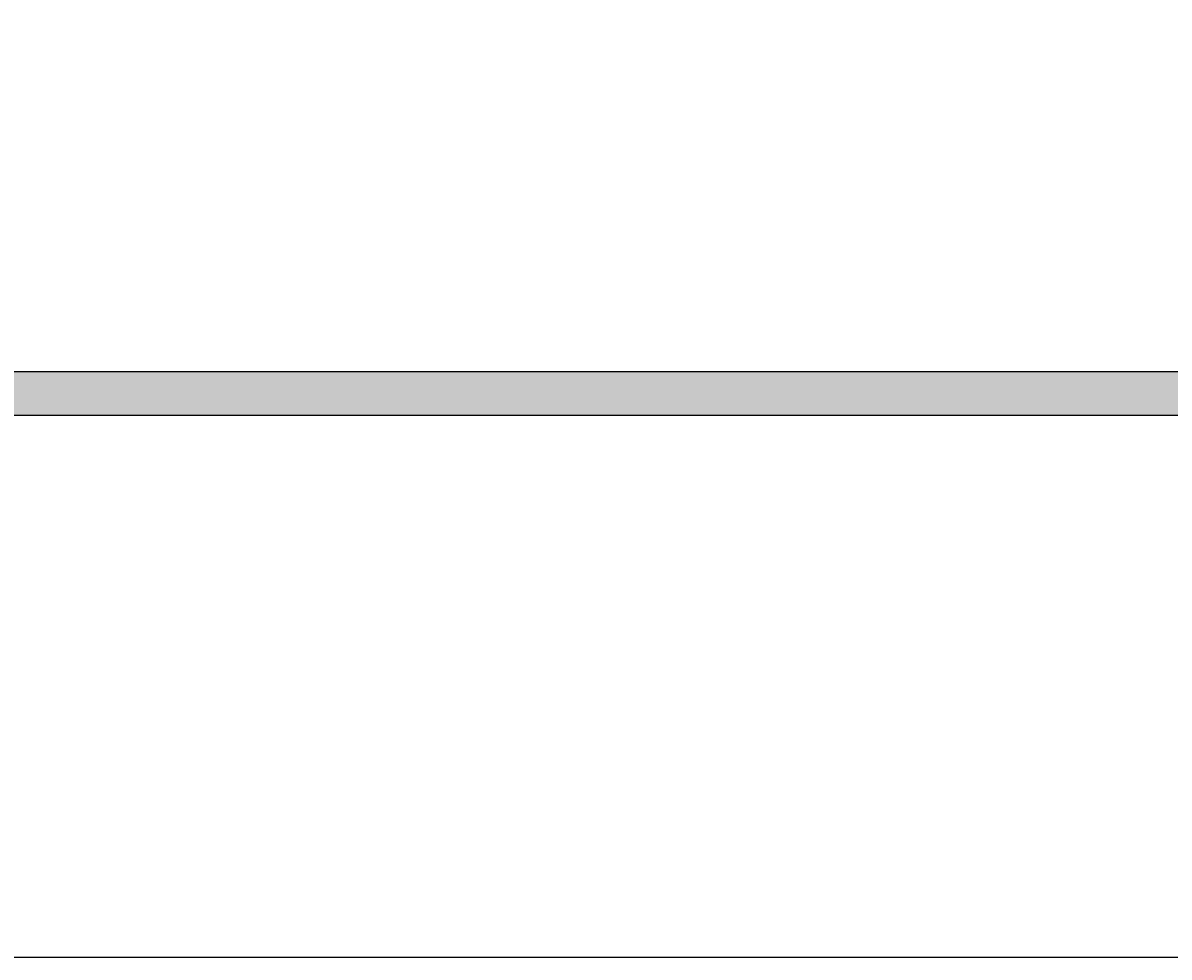
# Model space of a CAD drawing. Units: inches. Extents: x 35362 to 73946, y 43607 to 67532.
# Tile 133 of 134: x 69000 to 69530, y 45858 to 46290. Entities that reach past the tile are written whole.
import ezdxf

# ---------------------------------------------------------------- set-up
doc = ezdxf.new("R2010")
doc.units = ezdxf.units.IN
doc.header["$MEASUREMENT"] = 0
for name, color, linetype, lineweight in [('A-ANNO-DIMS', 2, 'Continuous', 18), ('E-SYMB', 1, 'Continuous', 25), ('E-SYMB-PATT', 1, 'Continuous', 13)]:
    doc.layers.add(name, color=color, linetype=linetype, lineweight=lineweight)
doc.styles.get("Standard").update_dxf_attribs({"font": 'arial.ttf'})
doc.dimstyles.get("Standard").update_dxf_attribs({"dimtxt": 0.18, "dimasz": 0.18, "dimexe": 0.18, "dimexo": 0.0625, "dimgap": 0.09, "dimtad": 0, "dimtih": 1, "dimtoh": 1, "dimdec": 4, "dimzin": 0, "dimdsep": 46, "dimtxsty": 'Standard', "dimcen": 0.09, "dimadec": 0, "dimazin": 0, "dimtfac": 1, "dimtdec": 4, "dimtofl": 0, "dimtmove": 0, "dimatfit": 3, "dimfxl": 1, "dimtolj": 1, "dimtzin": 0, "dimarcsym": 0})

# ---------------------------------------------------------------- blocks, each defined once
blk = doc.blocks.new('CT-CORE')
for p, q in [((-0.0004610742907971, 1387.996120092102), (-0.0004610742907971, -5.34733626409e-05)), ((19.9995389257092, -5.34733626409e-05), (19.99953892572375, 1387.996120092102))]:
    blk.add_line(p, q)
blk = doc.blocks.new('*D5')
at = {"layer": 'A-ANNO-DIMS', "color": 0, "lineweight": -2, "transparency": 16777216}
for p, q in [((37121.949085, 46919.318283), (37121.949085, 43606.678996)), ((69871.496302, 45449.831951), (69871.496302, 43606.678996)), ((37122.129085, 43606.858996), (53496.2943647142, 43606.858996)), ((69871.316302, 43606.858996), (53497.15102228581, 43606.858996))]:
    blk.add_line(p, q, dxfattribs=at)
at = {"layer": 'A-ANNO-DIMS', "color": 0, "transparency": 16777216}
for points in [[(37122.129085, 43606.888996), (37122.129085, 43606.828996), (37121.949085, 43606.858996)], [(69871.316302, 43606.888996), (69871.316302, 43606.828996), (69871.496302, 43606.858996)]]:
    blk.add_solid(points, dxfattribs=at)
at = {"layer": 'Defpoints', "color": 0, "transparency": 16777216}
for p in [(37121.949085, 46919.380783), (69871.496302, 45449.894451), (69871.496302, 43606.858996)]:
    blk.add_point(p, dxfattribs=at)
at = {"layer": 'A-ANNO-DIMS', "color": 0, "transparency": 16777216, "insert": (53496.7226935, 43606.858996), "char_height": 0.18, "attachment_point": 5}
blk.add_mtext('\\A1;32750', dxfattribs=at)
blk = doc.blocks.new('*D74')
at = {"layer": 'A-ANNO-DIMS', "color": 0, "lineweight": -2, "transparency": 16777216}
for p, q in [((55181.69646300003, 46108.87757800001), (73945.82566600003, 46108.87757800001)), ((73945.64566600005, 46108.69757800001), (73945.64566600005, 45983.7251866378)), ((73945.64566600005, 45858.38898900001), (73945.64566600005, 45983.36138036223)), ((55181.69646300003, 45858.20898900001), (73945.82566600003, 45858.20898900001))]:
    blk.add_line(p, q, dxfattribs=at)
at = {"layer": 'A-ANNO-DIMS', "color": 0, "transparency": 16777216}
for points in [[(73945.61566600006, 46108.69757800001), (73945.67566600005, 46108.69757800001), (73945.64566600005, 46108.87757800001)], [(73945.61566600006, 45858.38898900001), (73945.67566600005, 45858.38898900001), (73945.64566600005, 45858.20898900001)]]:
    blk.add_solid(points, dxfattribs=at)
at = {"layer": 'Defpoints', "color": 0, "transparency": 16777216}
for p in [(55181.63396300002, 46108.87757800001), (55181.63396300002, 45858.20898900001), (73945.64566600005, 45858.20898900001)]:
    blk.add_point(p, dxfattribs=at)
at = {"layer": 'A-ANNO-DIMS', "color": 0, "transparency": 16777216, "insert": (73945.64566600005, 45983.54328349999), "char_height": 0.18, "attachment_point": 5}
blk.add_mtext('\\A1;250.67', dxfattribs=at)

msp = doc.modelspace()

# ---------------------------------------------------------------- hatches: boundary and pattern name
at = {"layer": 'E-SYMB-PATT'}
h = msp.add_hatch(color=256, dxfattribs=at)
h.dxf.hatch_style = 1
h.paths.add_polyline_path([(69871.49630189747, 46108.87757831767), (69871.49630189747, 46128.87757831768), (68483.50012833202, 46128.87757831768), (68483.50012833202, 46108.87757831768)])

# ---------------------------------------------------------------- block references
at = {"layer": 'E-SYMB', "rotation": 269.9999999999974}
msp.add_blockref('CT-CORE', (68483.50018180539, 46128.87711724339), dxfattribs=at)

# ---------------------------------------------------------------- dimensions: what is measured, and where the dimension line sits
at = {"layer": 'A-ANNO-DIMS'}
dim = msp.add_linear_dim(base=(69871.496302, 43606.858996), p1=(37121.949085, 46919.380783), p2=(69871.496302, 45449.894451), dimstyle='Standard', override={"dimdec": 0, "dimlfac": 1, "dimrnd": 0, "dimzin": 0, "dimdsep": 46, "dimlunit": 2}, dxfattribs=at)
dim.commit()
dim.dimension.update_dxf_attribs({"geometry": '*D5', "text_midpoint": (53496.7226935, 43606.858996)})
dim = msp.add_linear_dim(base=(73945.64566600005, 45858.20898900001), p1=(55181.633963, 46108.877578), p2=(55181.633963, 45858.20898899999), angle=90, dimstyle='Standard', override={"dimdec": 2, "dimlfac": 1, "dimrnd": 0, "dimzin": 0, "dimdsep": 46, "dimlunit": 2}, dxfattribs=at)
dim.commit()
dim.dimension.update_dxf_attribs({"geometry": '*D74', "text_midpoint": (73945.64566600005, 45983.54328349999)})

doc.saveas('drawing.dxf')
